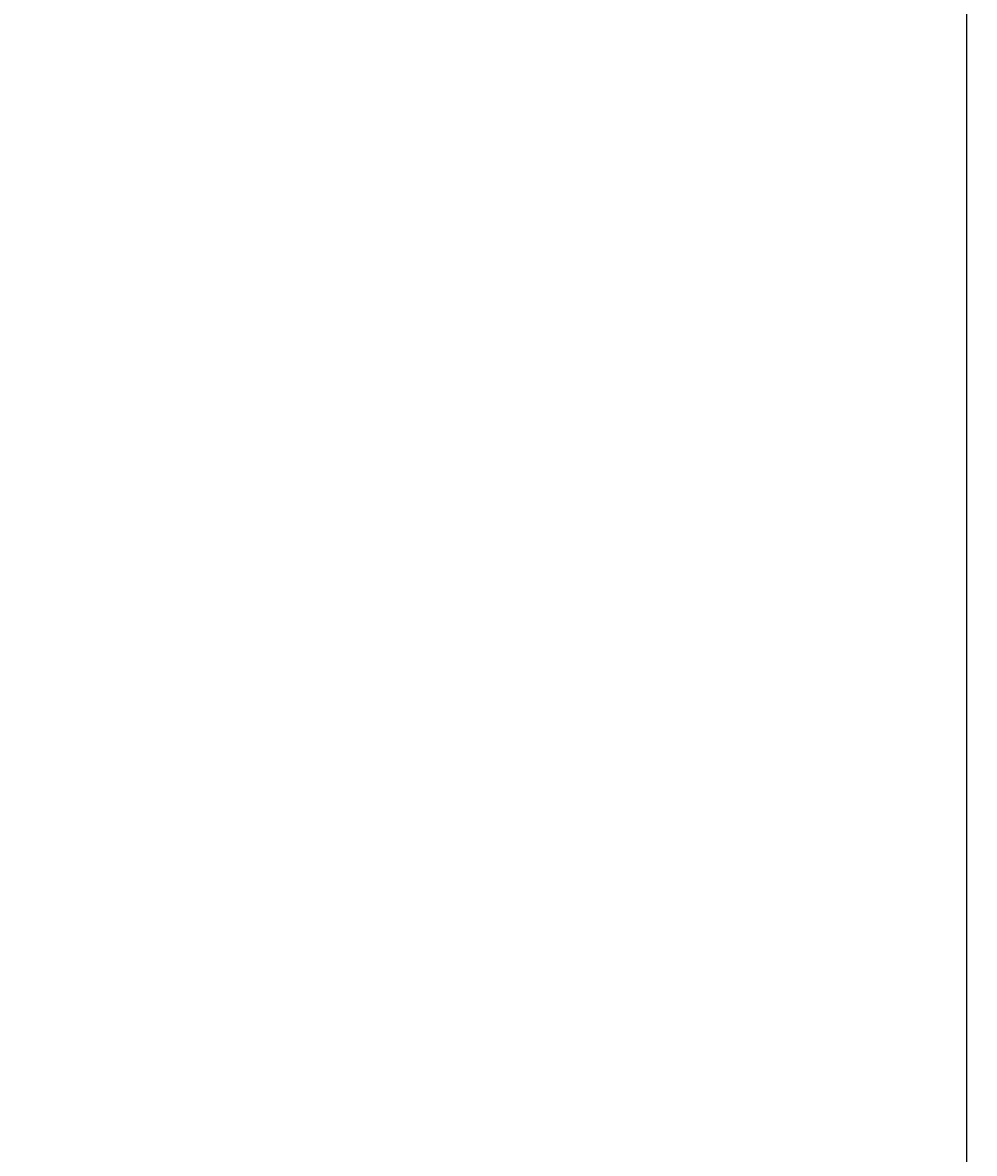
# Model space of a CAD drawing. Units: inches. Extents: x 1998 to 2588, y 1139 to 1977.
# Tile 116 of 134: x 2550 to 2588, y 1477 to 1523. Entities that reach past the tile are written whole.
import ezdxf

# ---------------------------------------------------------------- set-up
doc = ezdxf.new("R2010")
doc.units = ezdxf.units.IN
doc.layers.add('A-ANNO-DIMS', color=2, linetype='Continuous', lineweight=18)
doc.styles.get("Standard").update_dxf_attribs({"font": 'arial.ttf'})
doc.dimstyles.get("Standard").update_dxf_attribs({"dimtxt": 0.18, "dimasz": 0.18, "dimexe": 0.18, "dimexo": 0.0625, "dimgap": 0.09, "dimtad": 0, "dimtih": 1, "dimtoh": 1, "dimdec": 4, "dimzin": 0, "dimdsep": 46, "dimtxsty": 'Standard', "dimcen": 0.09, "dimadec": 0, "dimazin": 0, "dimtfac": 1, "dimtdec": 4, "dimtofl": 0, "dimtmove": 0, "dimatfit": 3, "dimfxl": 1, "dimtolj": 1, "dimtzin": 0, "dimarcsym": 0})

# ---------------------------------------------------------------- blocks, each defined once
blk = doc.blocks.new('*D24')
at = {"layer": 'A-ANNO-DIMS', "color": 0, "lineweight": -2, "transparency": 16777216}
for p, q in [((2398.535, 1911.232), (2588.309, 1911.232)), ((2588.129, 1911.052), (2588.129, 1570.164)), ((2588.129, 1228.912), (2588.129, 1569.8)), ((2527.535, 1228.732), (2588.309, 1228.732))]:
    blk.add_line(p, q, dxfattribs=at)
at = {"layer": 'A-ANNO-DIMS', "color": 0, "transparency": 16777216}
for points in [[(2588.099, 1911.052), (2588.159, 1911.052), (2588.129, 1911.232)], [(2588.099, 1228.912), (2588.159, 1228.912), (2588.129, 1228.732)]]:
    blk.add_solid(points, dxfattribs=at)
at = {"layer": 'Defpoints', "color": 0, "transparency": 16777216}
for p in [(2398.473, 1911.232), (2588.129, 1911.232), (2527.473, 1228.732)]:
    blk.add_point(p, dxfattribs=at)
at = {"layer": 'A-ANNO-DIMS', "color": 0, "transparency": 16777216, "insert": (2588.129, 1569.982), "char_height": 0.18, "attachment_point": 5}
blk.add_mtext('\\A1;682.5', dxfattribs=at)

msp = doc.modelspace()

# ---------------------------------------------------------------- dimensions: what is measured, and where the dimension line sits
at = {"layer": 'A-ANNO-DIMS'}
dim = msp.add_linear_dim(base=(2588.1286, 1911.2324), p1=(2527.4729, 1228.7324), p2=(2398.4729, 1911.2324), angle=90, dimstyle='Standard', override={"dimdec": 1, "dimlfac": 1, "dimrnd": 0, "dimzin": 0, "dimdsep": 46, "dimlunit": 2}, dxfattribs=at)
dim.commit()
dim.dimension.update_dxf_attribs({"geometry": '*D24', "text_midpoint": (2588.1286, 1569.9824)})

doc.saveas('drawing.dxf')
